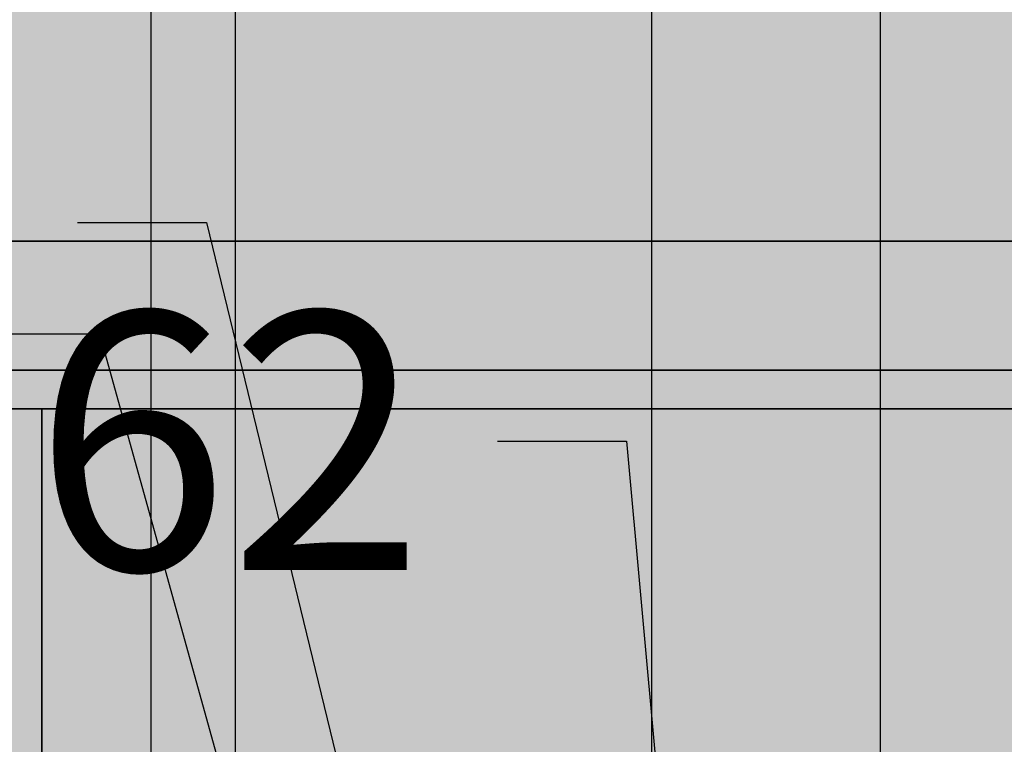
# Model space of a CAD drawing. Units: millimetres. Extents: x 130 to 1021, y 147 to 699.
# Tile 29 of 40: x 366 to 442, y 548 to 604. Entities that reach past the tile are written whole.
import ezdxf

# ---------------------------------------------------------------- set-up
doc = ezdxf.new("R2010")
doc.units = ezdxf.units.MM
doc.header["$MEASUREMENT"] = 0
for name, color, linetype, lineweight in [('A-ANNO-DIMS', 2, 'Continuous', 18), ('A-ELEV', 7, 'Continuous', 35), ('A-ELEV-PATT', 9, 'Continuous', 13)]:
    doc.layers.add(name, color=color, linetype=linetype, lineweight=lineweight)
doc.styles.get("Standard").update_dxf_attribs({"font": 'arial.ttf'})
doc.dimstyles.get("Standard").update_dxf_attribs({"dimtxt": 20, "dimasz": 10, "dimexe": 10, "dimexo": 10, "dimgap": 5, "dimtad": 0, "dimtih": 1, "dimtoh": 1, "dimdec": 0, "dimzin": 0, "dimdsep": 46, "dimtxsty": 'Standard', "dimcen": 5, "dimadec": 0, "dimazin": 0, "dimtfac": 1, "dimtdec": 0, "dimtofl": 0, "dimtmove": 0, "dimatfit": 3, "dimfxl": 1, "dimtolj": 1, "dimtzin": 0, "dimarcsym": 0})

# ---------------------------------------------------------------- blocks, each defined once
blk = doc.blocks.new('*D11')
at = {"layer": 'A-ANNO-DIMS', "color": 0, "lineweight": -2, "transparency": 16777216}
for p, q in [((737.374, 648.699), (737.374, 149.739)), ((299.374, 566.947), (299.374, 149.739)), ((309.374, 159.739), (490.857, 159.739)), ((727.374, 159.739), (545.891, 159.739))]:
    blk.add_line(p, q, dxfattribs=at)
at = {"layer": 'A-ANNO-DIMS', "color": 0, "transparency": 16777216}
for points in [[(309.374, 161.406), (309.374, 158.073), (299.374, 159.739)], [(727.374, 161.406), (727.374, 158.073), (737.374, 159.739)]]:
    blk.add_solid(points, dxfattribs=at)
at = {"layer": 'Defpoints', "color": 0, "transparency": 16777216}
for p in [(737.374, 658.699), (299.374, 576.947), (737.374, 159.739)]:
    blk.add_point(p, dxfattribs=at)
at = {"layer": 'A-ANNO-DIMS', "color": 0, "transparency": 16777216, "insert": (518.374, 159.739), "char_height": 20, "attachment_point": 5}
blk.add_mtext('\\A1;438', dxfattribs=at)
blk = doc.blocks.new('*D12')
at = {"layer": 'A-ANNO-DIMS', "color": 0, "lineweight": -2, "transparency": 16777216}
for p, q in [((477.374, 661.947), (265.074, 661.947)), ((275.074, 651.947), (275.074, 438.205)), ((275.074, 194.039), (275.074, 407.782)), ((357.163, 184.039), (265.074, 184.039))]:
    blk.add_line(p, q, dxfattribs=at)
at = {"layer": 'A-ANNO-DIMS', "color": 0, "transparency": 16777216}
for points in [[(273.407, 651.947), (276.74, 651.947), (275.074, 661.947)], [(273.407, 194.039), (276.74, 194.039), (275.074, 184.039)]]:
    blk.add_solid(points, dxfattribs=at)
at = {"layer": 'Defpoints', "color": 0, "transparency": 16777216}
for p in [(275.074, 661.947), (487.374, 661.947), (367.163, 184.039)]:
    blk.add_point(p, dxfattribs=at)
at = {"layer": 'A-ANNO-DIMS', "color": 0, "transparency": 16777216, "insert": (275.074, 422.993), "char_height": 20, "attachment_point": 5}
blk.add_mtext('\\A1;477.9', dxfattribs=at)
blk = doc.blocks.new('*D14')
at = {"layer": 'A-ANNO-DIMS', "color": 0, "lineweight": -2, "transparency": 16777216}
for p, q in [((307.374, 641.947), (307.374, 696.247)), ((327.374, 579.884), (327.374, 696.247)), ((297.374, 686.247), (287.374, 686.247)), ((337.374, 686.247), (347.374, 686.247))]:
    blk.add_line(p, q, dxfattribs=at)
at = {"layer": 'A-ANNO-DIMS', "color": 0, "transparency": 16777216}
for points in [[(297.374, 687.914), (297.374, 684.581), (307.374, 686.247)], [(337.374, 687.914), (337.374, 684.581), (327.374, 686.247)]]:
    blk.add_solid(points, dxfattribs=at)
at = {"layer": 'Defpoints', "color": 0, "transparency": 16777216}
for p in [(327.374, 686.247), (307.374, 631.947), (327.374, 569.884)]:
    blk.add_point(p, dxfattribs=at)
at = {"layer": 'A-ANNO-DIMS', "color": 0, "transparency": 16777216, "insert": (366.835, 686.247), "char_height": 20, "attachment_point": 5}
blk.add_mtext('\\A1;20', dxfattribs=at)
blk = doc.blocks.new('*D15')
at = {"layer": 'A-ANNO-DIMS', "color": 0, "lineweight": -2, "transparency": 16777216}
for p, q in [((327.374, 579.884), (327.374, 696.247)), ((357.941, 411.947), (357.941, 696.247)), ((337.374, 686.247), (347.941, 686.247)), ((357.941, 686.247), (367.941, 686.247))]:
    blk.add_line(p, q, dxfattribs=at)
at = {"layer": 'A-ANNO-DIMS', "color": 0, "transparency": 16777216}
for points in [[(337.374, 687.914), (337.374, 684.581), (327.374, 686.247)], [(347.941, 687.914), (347.941, 684.581), (357.941, 686.247)]]:
    blk.add_solid(points, dxfattribs=at)
at = {"layer": 'Defpoints', "color": 0, "transparency": 16777216}
for p in [(357.941, 686.247), (327.374, 569.884), (357.941, 401.947)]:
    blk.add_point(p, dxfattribs=at)
at = {"layer": 'A-ANNO-DIMS', "color": 0, "transparency": 16777216, "insert": (406.679, 686.247), "char_height": 20, "attachment_point": 5}
blk.add_mtext('\\A1;30.57', dxfattribs=at)
blk = doc.blocks.new('*D16')
at = {"layer": 'A-ANNO-DIMS', "color": 0, "lineweight": -2, "transparency": 16777216}
for p, q in [((357.941, 411.947), (357.941, 696.247)), ((363.922, 579.884), (363.922, 696.247)), ((347.941, 686.247), (337.941, 686.247)), ((373.922, 686.247), (383.922, 686.247))]:
    blk.add_line(p, q, dxfattribs=at)
at = {"layer": 'A-ANNO-DIMS', "color": 0, "transparency": 16777216}
for points in [[(347.941, 687.914), (347.941, 684.581), (357.941, 686.247)], [(373.922, 687.914), (373.922, 684.581), (363.922, 686.247)]]:
    blk.add_solid(points, dxfattribs=at)
at = {"layer": 'Defpoints', "color": 0, "transparency": 16777216}
for p in [(363.922, 686.247), (363.922, 569.884), (357.941, 401.947)]:
    blk.add_point(p, dxfattribs=at)
at = {"layer": 'A-ANNO-DIMS', "color": 0, "transparency": 16777216, "insert": (420.737, 686.247), "char_height": 20, "attachment_point": 5}
blk.add_mtext('\\A1;5.981', dxfattribs=at)
blk = doc.blocks.new('*D17')
at = {"layer": 'A-ANNO-DIMS', "color": 0, "lineweight": -2, "transparency": 16777216}
for p, q in [((363.922, 579.884), (363.922, 696.247)), ((375.85, 490.216), (375.85, 696.247)), ((353.922, 686.247), (343.922, 686.247)), ((385.85, 686.247), (395.85, 686.247))]:
    blk.add_line(p, q, dxfattribs=at)
at = {"layer": 'A-ANNO-DIMS', "color": 0, "transparency": 16777216}
for points in [[(353.922, 687.914), (353.922, 684.581), (363.922, 686.247)], [(385.85, 687.914), (385.85, 684.581), (375.85, 686.247)]]:
    blk.add_solid(points, dxfattribs=at)
at = {"layer": 'Defpoints', "color": 0, "transparency": 16777216}
for p in [(375.85, 686.247), (363.922, 569.884), (375.85, 480.216)]:
    blk.add_point(p, dxfattribs=at)
at = {"layer": 'A-ANNO-DIMS', "color": 0, "transparency": 16777216, "insert": (441.444, 686.247), "char_height": 20, "attachment_point": 5}
blk.add_mtext('\\A1;11.928', dxfattribs=at)
blk = doc.blocks.new('*D18')
at = {"layer": 'A-ANNO-DIMS', "color": 0, "lineweight": -2, "transparency": 16777216}
for p, q in [((375.85, 490.216), (375.85, 696.247)), ((382.374, 388.947), (382.374, 696.247)), ((365.85, 686.247), (355.85, 686.247)), ((392.374, 686.247), (402.374, 686.247))]:
    blk.add_line(p, q, dxfattribs=at)
at = {"layer": 'A-ANNO-DIMS', "color": 0, "transparency": 16777216}
for points in [[(365.85, 687.914), (365.85, 684.581), (375.85, 686.247)], [(392.374, 687.914), (392.374, 684.581), (382.374, 686.247)]]:
    blk.add_solid(points, dxfattribs=at)
at = {"layer": 'Defpoints', "color": 0, "transparency": 16777216}
for p in [(382.374, 686.247), (375.85, 480.216), (382.374, 378.947)]:
    blk.add_point(p, dxfattribs=at)
at = {"layer": 'A-ANNO-DIMS', "color": 0, "transparency": 16777216, "insert": (441.132, 686.247), "char_height": 20, "attachment_point": 5}
blk.add_mtext('\\A1;6.524', dxfattribs=at)
blk = doc.blocks.new('*D19')
at = {"layer": 'A-ANNO-DIMS', "color": 0, "lineweight": -2, "transparency": 16777216}
for p, q in [((382.374, 388.947), (382.374, 696.247)), ((414.652, 510.881), (414.652, 696.247)), ((392.374, 686.247), (404.652, 686.247)), ((414.652, 686.247), (424.652, 686.247))]:
    blk.add_line(p, q, dxfattribs=at)
at = {"layer": 'A-ANNO-DIMS', "color": 0, "transparency": 16777216}
for points in [[(392.374, 687.914), (392.374, 684.581), (382.374, 686.247)], [(404.652, 687.914), (404.652, 684.581), (414.652, 686.247)]]:
    blk.add_solid(points, dxfattribs=at)
at = {"layer": 'Defpoints', "color": 0, "transparency": 16777216}
for p in [(414.652, 686.247), (414.652, 500.881), (382.374, 378.947)]:
    blk.add_point(p, dxfattribs=at)
at = {"layer": 'A-ANNO-DIMS', "color": 0, "transparency": 16777216, "insert": (463.411, 686.247), "char_height": 20, "attachment_point": 5}
blk.add_mtext('\\A1;32.28', dxfattribs=at)
blk = doc.blocks.new('*D20')
at = {"layer": 'A-ANNO-DIMS', "color": 0, "lineweight": -2, "transparency": 16777216}
for p, q in [((414.652, 510.881), (414.652, 696.247)), ((432.374, 388.947), (432.374, 696.247)), ((404.652, 686.247), (394.652, 686.247)), ((442.374, 686.247), (452.374, 686.247))]:
    blk.add_line(p, q, dxfattribs=at)
at = {"layer": 'A-ANNO-DIMS', "color": 0, "transparency": 16777216}
for points in [[(404.652, 687.914), (404.652, 684.581), (414.652, 686.247)], [(442.374, 687.914), (442.374, 684.581), (432.374, 686.247)]]:
    blk.add_solid(points, dxfattribs=at)
at = {"layer": 'Defpoints', "color": 0, "transparency": 16777216}
for p in [(432.374, 686.247), (414.652, 500.881), (432.374, 378.947)]:
    blk.add_point(p, dxfattribs=at)
at = {"layer": 'A-ANNO-DIMS', "color": 0, "transparency": 16777216, "insert": (490.075, 686.247), "char_height": 20, "attachment_point": 5}
blk.add_mtext('\\A1;17.72', dxfattribs=at)
blk = doc.blocks.new('*D21')
at = {"layer": 'A-ANNO-DIMS', "color": 0, "lineweight": -2, "transparency": 16777216}
for p, q in [((432.374, 388.947), (432.374, 696.247)), ((447.374, 656.947), (447.374, 696.247)), ((422.374, 686.247), (412.374, 686.247)), ((457.374, 686.247), (467.374, 686.247))]:
    blk.add_line(p, q, dxfattribs=at)
at = {"layer": 'A-ANNO-DIMS', "color": 0, "transparency": 16777216}
for points in [[(422.374, 687.914), (422.374, 684.581), (432.374, 686.247)], [(457.374, 687.914), (457.374, 684.581), (447.374, 686.247)]]:
    blk.add_solid(points, dxfattribs=at)
at = {"layer": 'Defpoints', "color": 0, "transparency": 16777216}
for p in [(447.374, 686.247), (447.374, 646.947), (432.374, 378.947)]:
    blk.add_point(p, dxfattribs=at)
at = {"layer": 'A-ANNO-DIMS', "color": 0, "transparency": 16777216, "insert": (485.832, 686.247), "char_height": 20, "attachment_point": 5}
blk.add_mtext('\\A1;15', dxfattribs=at)
blk = doc.blocks.new('*D22')
at = {"layer": 'A-ANNO-DIMS', "color": 0, "lineweight": -2, "transparency": 16777216}
for p, q in [((447.374, 656.947), (447.374, 696.247)), ((466.767, 403.947), (466.767, 696.247)), ((437.374, 686.247), (427.374, 686.247)), ((476.767, 686.247), (486.767, 686.247))]:
    blk.add_line(p, q, dxfattribs=at)
at = {"layer": 'A-ANNO-DIMS', "color": 0, "transparency": 16777216}
for points in [[(437.374, 687.914), (437.374, 684.581), (447.374, 686.247)], [(476.767, 687.914), (476.767, 684.581), (466.767, 686.247)]]:
    blk.add_solid(points, dxfattribs=at)
at = {"layer": 'Defpoints', "color": 0, "transparency": 16777216}
for p in [(466.767, 686.247), (447.374, 646.947), (466.767, 393.947)]:
    blk.add_point(p, dxfattribs=at)
at = {"layer": 'A-ANNO-DIMS', "color": 0, "transparency": 16777216, "insert": (532.34, 686.247), "char_height": 20, "attachment_point": 5}
blk.add_mtext('\\A1;19.393', dxfattribs=at)
blk = doc.blocks.new('*D44')
at = {"layer": 'A-ANNO-DIMS', "color": 0, "lineweight": -2, "transparency": 16777216}
for p, q in [((317.374, 569.884), (265.074, 569.884)), ((275.074, 559.884), (275.074, 550.594)), ((275.074, 510.881), (275.074, 520.171)), ((404.652, 500.881), (265.074, 500.881))]:
    blk.add_line(p, q, dxfattribs=at)
at = {"layer": 'A-ANNO-DIMS', "color": 0, "transparency": 16777216}
for points in [[(273.407, 559.884), (276.74, 559.884), (275.074, 569.884)], [(273.407, 510.881), (276.74, 510.881), (275.074, 500.881)]]:
    blk.add_solid(points, dxfattribs=at)
at = {"layer": 'Defpoints', "color": 0, "transparency": 16777216}
for p in [(275.074, 569.884), (327.374, 569.884), (414.652, 500.881)]:
    blk.add_point(p, dxfattribs=at)
at = {"layer": 'A-ANNO-DIMS', "color": 0, "transparency": 16777216, "insert": (275.074, 535.383), "char_height": 20, "attachment_point": 5}
blk.add_mtext('\\A1;69', dxfattribs=at)
blk = doc.blocks.new('*D66')
at = {"layer": 'A-ANNO-DIMS', "color": 0, "lineweight": -2, "transparency": 16777216}
for p, q in [((341.579, 557.194), (351.579, 557.194)), ((351.579, 557.194), (376.947, 478.135)), ((427.374, 315.978), (427.374, 325.978)), ((422.374, 320.978), (432.374, 320.978))]:
    blk.add_line(p, q, dxfattribs=at)
at = {"layer": 'A-ANNO-DIMS', "color": 0, "transparency": 16777216}
blk.add_solid([(378.534, 478.644), (375.36, 477.626), (380.002, 468.613)], dxfattribs=at)
at = {"layer": 'Defpoints', "color": 0, "transparency": 16777216}
for p in [(380.002, 468.613), (427.374, 320.978)]:
    blk.add_point(p, dxfattribs=at)
at = {"layer": 'A-ANNO-DIMS', "color": 0, "transparency": 16777216, "insert": (263.53, 557.194), "char_height": 20, "attachment_point": 5}
blk.add_mtext('\\A1;4X R155.05', dxfattribs=at)
blk = doc.blocks.new('*D68')
at = {"layer": 'A-ANNO-DIMS', "color": 0, "lineweight": -2, "transparency": 16777216}
for p, q in [((361.841, 579.756), (371.841, 579.756)), ((371.841, 579.756), (392.167, 506.693)), ((433.191, 354.23), (433.191, 364.23)), ((428.191, 359.23), (438.191, 359.23))]:
    blk.add_line(p, q, dxfattribs=at)
at = {"layer": 'A-ANNO-DIMS', "color": 0, "transparency": 16777216}
blk.add_solid([(393.773, 507.14), (390.561, 506.246), (394.847, 497.059)], dxfattribs=at)
at = {"layer": 'Defpoints', "color": 0, "transparency": 16777216}
for p in [(394.847, 497.059), (433.191, 359.23)]:
    blk.add_point(p, dxfattribs=at)
at = {"layer": 'A-ANNO-DIMS', "color": 0, "transparency": 16777216, "insert": (305.764, 579.756), "char_height": 20, "attachment_point": 5}
blk.add_mtext('\\A1;R143.06', dxfattribs=at)
blk = doc.blocks.new('*D69')
at = {"layer": 'A-ANNO-DIMS', "color": 0, "lineweight": -2, "transparency": 16777216}
for p, q in [((507.746, 572.261), (483.091, 501.813)), ((517.746, 572.261), (507.746, 572.261)), ((433.191, 354.23), (433.191, 364.23)), ((428.191, 359.23), (438.191, 359.23))]:
    blk.add_line(p, q, dxfattribs=at)
at = {"layer": 'A-ANNO-DIMS', "color": 0, "transparency": 16777216}
blk.add_solid([(481.518, 502.363), (484.664, 501.262), (479.788, 492.374)], dxfattribs=at)
at = {"layer": 'Defpoints', "color": 0, "transparency": 16777216}
for p in [(479.788, 492.374), (433.191, 359.23)]:
    blk.add_point(p, dxfattribs=at)
at = {"layer": 'A-ANNO-DIMS', "color": 0, "transparency": 16777216, "insert": (573.824, 572.261), "char_height": 20, "attachment_point": 5}
blk.add_mtext('\\A1;R141.06', dxfattribs=at)
blk = doc.blocks.new('*D70')
at = {"layer": 'A-ANNO-DIMS', "color": 0, "lineweight": -2, "transparency": 16777216}
for p, q in [((370.141, 588.4), (380.141, 588.4)), ((380.141, 588.4), (397.473, 517.008)), ((432.65, 367.109), (432.65, 377.109)), ((427.65, 372.109), (437.65, 372.109))]:
    blk.add_line(p, q, dxfattribs=at)
at = {"layer": 'A-ANNO-DIMS', "color": 0, "transparency": 16777216}
blk.add_solid([(399.093, 517.402), (395.854, 516.615), (399.832, 507.291)], dxfattribs=at)
at = {"layer": 'Defpoints', "color": 0, "transparency": 16777216}
for p in [(399.832, 507.291), (432.65, 372.109)]:
    blk.add_point(p, dxfattribs=at)
at = {"layer": 'A-ANNO-DIMS', "color": 0, "transparency": 16777216, "insert": (323.757, 588.4), "char_height": 20, "attachment_point": 5}
blk.add_mtext('\\A1;R139.1', dxfattribs=at)
blk = doc.blocks.new('*D71')
at = {"layer": 'A-ANNO-DIMS', "color": 0, "lineweight": -2, "transparency": 16777216}
for p, q in [((492.108, 581.609), (472.542, 512.666)), ((502.108, 581.609), (492.108, 581.609)), ((432.65, 367.109), (432.65, 377.109)), ((427.65, 372.109), (437.65, 372.109))]:
    blk.add_line(p, q, dxfattribs=at)
at = {"layer": 'A-ANNO-DIMS', "color": 0, "transparency": 16777216}
blk.add_solid([(470.938, 513.121), (474.145, 512.211), (469.812, 503.046)], dxfattribs=at)
at = {"layer": 'Defpoints', "color": 0, "transparency": 16777216}
for p in [(469.812, 503.046), (432.65, 372.109)]:
    blk.add_point(p, dxfattribs=at)
at = {"layer": 'A-ANNO-DIMS', "color": 0, "transparency": 16777216, "insert": (548.493, 581.609), "char_height": 20, "attachment_point": 5}
blk.add_mtext('\\A1;R136.1', dxfattribs=at)
blk = doc.blocks.new('*D72')
at = {"layer": 'A-ANNO-DIMS', "color": 0, "lineweight": -2, "transparency": 16777216}
for p, q in [((460.658, 573.64), (451.279, 503.49)), ((470.658, 573.64), (460.658, 573.64)), ((432.115, 355.142), (432.115, 365.142)), ((427.115, 360.142), (437.115, 360.142))]:
    blk.add_line(p, q, dxfattribs=at)
at = {"layer": 'A-ANNO-DIMS', "color": 0, "transparency": 16777216}
blk.add_solid([(449.628, 503.711), (452.931, 503.27), (449.954, 493.579)], dxfattribs=at)
at = {"layer": 'Defpoints', "color": 0, "transparency": 16777216}
for p in [(449.954, 493.579), (432.115, 360.142)]:
    blk.add_point(p, dxfattribs=at)
at = {"layer": 'A-ANNO-DIMS', "color": 0, "transparency": 16777216, "insert": (526.64, 573.64), "char_height": 20, "attachment_point": 5}
blk.add_mtext('\\A1;R134.62', dxfattribs=at)
blk = doc.blocks.new('*D73')
at = {"layer": 'A-ANNO-DIMS', "color": 0, "lineweight": -2, "transparency": 16777216}
for p, q in [((402.678, 571.448), (412.678, 571.448)), ((412.678, 571.448), (419.051, 502.166)), ((432.115, 355.142), (432.115, 365.142)), ((427.115, 360.142), (437.115, 360.142))]:
    blk.add_line(p, q, dxfattribs=at)
at = {"layer": 'A-ANNO-DIMS', "color": 0, "transparency": 16777216}
blk.add_solid([(420.711, 502.319), (417.391, 502.014), (419.967, 492.208)], dxfattribs=at)
at = {"layer": 'Defpoints', "color": 0, "transparency": 16777216}
for p in [(419.967, 492.208), (432.115, 360.142)]:
    blk.add_point(p, dxfattribs=at)
at = {"layer": 'A-ANNO-DIMS', "color": 0, "transparency": 16777216, "insert": (346.696, 571.448), "char_height": 20, "attachment_point": 5}
blk.add_mtext('\\A1;R132.62', dxfattribs=at)

msp = doc.modelspace()

# ---------------------------------------------------------------- hatches: boundary and pattern name
at = {"layer": 'A-ELEV-PATT'}
h = msp.add_hatch(color=256, dxfattribs=at)
h.dxf.hatch_style = 1
h.paths.add_polyline_path([(737.3738, 658.6988, 0.0135961), (632.4019, 661.9473), (607.3738, 661.9473), (487.3738, 661.9473), (487.3738, 649.9473), (607.3738, 649.9473), (632.3794, 649.9473, -0.0136841), (737.3738, 646.6784)])
h.paths.add_polyline_path([(732.3738, 643.9599, 0.0130529), (632.3738, 646.9473), (607.3738, 646.9473), (487.3738, 646.9473), (487.3738, 596.9473), (632.3738, 596.9473, -0.0130529), (732.3738, 593.9599)])
h.paths.add_polyline_path([(737.3738, 593.6732, 0.0137063), (632.3738, 596.9473), (487.3738, 596.9473), (487.3738, 586.9473), (632.355, 586.9473, -0.0137808), (737.3738, 583.6559)])
h.paths.add_polyline_path([(447.3738, 646.9473), (307.3738, 646.9473), (302.3738, 646.9473), (302.3738, 634.9473), (447.3738, 634.9473)])
h.paths.add_polyline_path([(447.3738, 631.9473), (307.3738, 631.9473), (307.3738, 586.9473), (447.3738, 586.9473)])
h.paths.add_polyline_path([(447.3738, 586.9473), (307.3738, 586.9473), (302.3738, 586.9473), (302.3738, 576.9473), (447.3738, 576.9473)])
h.paths.add_polyline_path([(447.3738, 573.9473), (367.3738, 573.9473), (367.3738, 539.9473), (447.3738, 539.9473)])
h.paths.add_polyline_path([(447.3738, 537.9473), (367.3738, 537.9473), (367.3738, 507.9473), (400.392, 507.4253, -0.001728), (401.3281, 507.6451, -0.5220025), (425.6117, 511.0391, -0.0391849), (447.3738, 510.4359), (447.3738, 510.7883)])
h.paths.add_polyline_path([(394.7238, 505.9473), (367.3738, 505.9473), (367.3738, 476.9473, -0.0146512), (375.8501, 480.2159), (376.1506, 499.2266, -0.0355419)])
h.paths.add_polyline_path([(632.3738, 583.9473), (552.3738, 583.9473), (552.3738, 550.9473), (632.3738, 550.9473)])
h.paths.add_polyline_path([(632.3738, 548.9473), (552.3738, 548.9473), (552.3738, 515.9473), (632.3738, 515.9473)])
h.paths.add_polyline_path([(632.3738, 513.9473), (552.3738, 513.9473), (552.3738, 476.9473), (632.3738, 476.9473)])
h.paths.add_polyline_path([(737.3738, 473.6903, 0.0136326), (632.3926, 476.9473), (552.3738, 476.9473), (487.3738, 476.9473), (487.3738, 466.9473), (632.3738, 466.9473, -0.0137063), (737.3738, 463.6732)])
h.paths.add_polyline_path([(732.3738, 460.9552, 0.0130741), (632.3681, 463.9473), (487.3738, 463.9473), (487.3738, 407.735, -0.0032286), (489.3544, 406.9473), (632.3926, 406.9473, -0.0129826), (732.3738, 403.9755)])
h.paths.add_polyline_path([(487.3738, 463.9473, 0.20133), (367.3738, 463.9473), (367.3738, 407.735, -0.1882031), (487.3738, 407.735)])
h.paths.add_polyline_path([(367.3738, 476.9473), (367.3738, 466.9473, -0.2013309), (487.3738, 466.9473), (487.3738, 476.9473, 0.20133)])
h.paths.add_polyline_path([(367.3738, 463.9473), (307.3738, 463.9473), (307.3738, 401.9473), (357.9413, 401.9473), (367.3738, 407.735)])
h.paths.add_polyline_path([(367.3738, 476.9473), (302.3738, 476.9473), (302.3738, 466.9473), (367.3738, 466.9473)])
h.paths.add_polyline_path([(632.8184, 366.9453), (552.3738, 366.9453), (552.3738, 393.9473), (632.8184, 393.9473)])
h.paths.add_polyline_path([(632.8184, 357.2114), (632.8184, 363.9453), (552.3738, 363.9453), (552.3738, 357.2114), (552.3738, 336.9453), (632.8184, 336.9453)])
h.paths.add_polyline_path([(632.8184, 333.9453), (552.3738, 333.9453), (552.3738, 306.9453), (632.8184, 306.9453)])
h.paths.add_polyline_path([(632.8184, 303.9453), (552.3738, 303.9453), (552.3738, 273.9473), (632.355, 273.9473, 0.0000608), (632.8184, 273.9491)])
h.paths.add_polyline_path([(737.3738, 403.6903, 0.0136326), (632.3926, 406.9473), (489.3544, 406.9473, 0.1915481), (367.3738, 407.735), (367.3738, 396.9473, -0.2013309), (487.3738, 396.9473), (632.3738, 396.9473, -0.0137063), (737.3738, 393.6732)])
h.paths.add_polyline_path([(357.9413, 401.9473), (307.3738, 401.9473), (307.3738, 391.9473), (357.9413, 391.9473)])
h.paths.add_polyline_path([(357.9413, 357.2114), (357.9413, 388.9473), (307.3738, 388.9473), (307.3738, 357.2114), (307.3738, 273.9473), (357.9413, 273.9473)])
h.paths.add_polyline_path([(732.3738, 263.93, -0.0130317), (632.3794, 260.9473), (466.7667, 260.9473), (466.7667, 240.9473), (469.8406, 236.978), (469.8406, 221.978), (472.9145, 218.0087), (472.9145, 213.9473), (607.3738, 213.9473), (732.3738, 213.9473)])
h.paths.add_polyline_path([(732.3738, 290.889), (722.479, 290.889), (722.479, 301.889), (732.3738, 301.889), (732.3738, 305.889), (722.479, 305.889), (722.479, 316.889), (732.3738, 316.889), (732.3738, 320.889), (722.479, 320.889), (722.479, 331.889), (732.3738, 331.889), (732.3738, 335.889), (722.479, 335.889), (722.479, 346.889), (732.3738, 346.889), (732.3738, 350.889), (722.479, 350.889), (722.479, 361.889), (732.3738, 361.889), (732.3738, 365.889), (722.479, 365.889), (722.479, 376.889), (732.3738, 376.889), (732.3738, 380.889), (722.479, 380.889), (722.479, 391.4848, 0.0005233), (718.479, 391.6843), (718.479, 380.889), (707.479, 380.889), (707.479, 392.1896, 0.0005231), (703.479, 392.3576), (703.479, 380.889), (692.479, 380.889), (692.479, 392.7765, 0.0005229), (688.479, 392.9131), (688.479, 380.889), (677.479, 380.889), (677.479, 393.2456, 0.0005228), (673.479, 393.3508), (673.479, 380.889), (662.479, 380.889), (662.479, 393.597, 0.0005227), (658.479, 393.6709), (658.479, 380.889), (647.479, 380.889), (647.479, 393.8308, 0.0005226), (643.479, 393.8732), (643.479, 380.889), (632.8184, 380.889), (632.8184, 376.889), (643.479, 376.889), (643.479, 365.889), (632.8184, 365.889), (632.8184, 361.889), (643.479, 361.889), (643.479, 350.889), (632.8184, 350.889), (632.8184, 346.889), (643.479, 346.889), (643.479, 335.889), (632.8184, 335.889), (632.8184, 331.889), (643.479, 331.889), (643.479, 320.889), (632.8184, 320.889), (632.8184, 316.889), (643.479, 316.889), (643.479, 305.889), (632.8184, 305.889), (632.8184, 301.889), (643.479, 301.889), (643.479, 290.889), (632.8184, 290.889), (632.8184, 286.889), (643.479, 286.889), (643.479, 274.0217, 0.0005246), (647.479, 274.0643), (647.479, 286.889), (658.479, 286.889), (658.479, 274.2248, 0.0005246), (662.479, 274.2989), (662.479, 286.889), (673.479, 286.889), (673.479, 274.546, 0.0005247), (677.479, 274.6516), (677.479, 286.889), (688.479, 286.889), (688.479, 274.9853, 0.0005248), (692.479, 275.1224), (692.479, 286.889), (703.479, 286.889), (703.479, 275.5429, 0.000525), (707.479, 275.7115), (707.479, 286.889), (718.479, 286.889), (718.479, 276.2187, 0.0005252), (722.479, 276.4189), (722.479, 286.889), (732.3738, 286.889)])
h.paths.add_polyline_path([(718.479, 290.889), (707.479, 290.889), (707.479, 301.889), (718.479, 301.889)], flags=16)
h.paths.add_polyline_path([(703.479, 290.889), (692.479, 290.889), (692.479, 301.889), (703.479, 301.889)], flags=16)
h.paths.add_polyline_path([(718.479, 305.889), (707.479, 305.889), (707.479, 316.889), (718.479, 316.889)], flags=16)
h.paths.add_polyline_path([(703.479, 305.889), (692.479, 305.889), (692.479, 316.889), (703.479, 316.889)], flags=16)
h.paths.add_polyline_path([(688.479, 290.889), (677.479, 290.889), (677.479, 301.889), (688.479, 301.889)], flags=16)
h.paths.add_polyline_path([(718.479, 320.889), (707.479, 320.889), (707.479, 331.889), (718.479, 331.889)], flags=16)
h.paths.add_polyline_path([(688.479, 305.889), (677.479, 305.889), (677.479, 316.889), (688.479, 316.889)], flags=16)
h.paths.add_polyline_path([(703.479, 320.889), (692.479, 320.889), (692.479, 331.889), (703.479, 331.889)], flags=16)
h.paths.add_polyline_path([(688.479, 320.889), (677.479, 320.889), (677.479, 331.889), (688.479, 331.889)], flags=16)
h.paths.add_polyline_path([(673.479, 290.889), (662.479, 290.889), (662.479, 301.889), (673.479, 301.889)], flags=16)
h.paths.add_polyline_path([(718.479, 335.889), (707.479, 335.889), (707.479, 346.889), (718.479, 346.889)], flags=16)
h.paths.add_polyline_path([(673.479, 305.889), (662.479, 305.889), (662.479, 316.889), (673.479, 316.889)], flags=16)
h.paths.add_polyline_path([(703.479, 335.889), (692.479, 335.889), (692.479, 346.889), (703.479, 346.889)], flags=16)
h.paths.add_polyline_path([(673.479, 320.889), (662.479, 320.889), (662.479, 331.889), (673.479, 331.889)], flags=16)
h.paths.add_polyline_path([(688.479, 335.889), (677.479, 335.889), (677.479, 346.889), (688.479, 346.889)], flags=16)
h.paths.add_polyline_path([(658.479, 290.889), (647.479, 290.889), (647.479, 301.889), (658.479, 301.889)], flags=16)
h.paths.add_polyline_path([(718.479, 350.889), (707.479, 350.889), (707.479, 361.889), (718.479, 361.889)], flags=16)
h.paths.add_polyline_path([(658.479, 305.889), (647.479, 305.889), (647.479, 316.889), (658.479, 316.889)], flags=16)
h.paths.add_polyline_path([(703.479, 350.889), (692.479, 350.889), (692.479, 361.889), (703.479, 361.889)], flags=16)
h.paths.add_polyline_path([(673.479, 335.889), (662.479, 335.889), (662.479, 346.889), (673.479, 346.889)], flags=16)
h.paths.add_polyline_path([(658.479, 320.889), (647.479, 320.889), (647.479, 331.889), (658.479, 331.889)], flags=16)
h.paths.add_polyline_path([(688.479, 350.889), (677.479, 350.889), (677.479, 361.889), (688.479, 361.889)], flags=16)
h.paths.add_polyline_path([(718.479, 365.889), (707.479, 365.889), (707.479, 376.889), (718.479, 376.889)], flags=16)
h.paths.add_polyline_path([(658.479, 335.889), (647.479, 335.889), (647.479, 346.889), (658.479, 346.889)], flags=16)
h.paths.add_polyline_path([(673.479, 350.889), (662.479, 350.889), (662.479, 361.889), (673.479, 361.889)], flags=16)
h.paths.add_polyline_path([(703.479, 365.889), (692.479, 365.889), (692.479, 376.889), (703.479, 376.889)], flags=16)
h.paths.add_polyline_path([(688.479, 365.889), (677.479, 365.889), (677.479, 376.889), (688.479, 376.889)], flags=16)
h.paths.add_polyline_path([(658.479, 350.889), (647.479, 350.889), (647.479, 361.889), (658.479, 361.889)], flags=16)
h.paths.add_polyline_path([(673.479, 365.889), (662.479, 365.889), (662.479, 376.889), (673.479, 376.889)], flags=16)
h.paths.add_polyline_path([(658.479, 365.889), (647.479, 365.889), (647.479, 376.889), (658.479, 376.889)], flags=16)
h.paths.add_polyline_path([(732.3738, 503.9786), (722.3392, 503.9786), (722.3392, 514.9786), (732.3738, 514.9786), (732.3738, 518.9786), (722.3392, 518.9786), (722.3392, 529.9786), (732.3738, 529.9786), (732.3738, 533.9786), (722.3392, 533.9786), (722.3392, 544.9786), (732.3738, 544.9786), (732.3738, 546.9473), (732.3738, 548.9786), (722.3392, 548.9786), (722.3392, 559.9786), (732.3738, 559.9786), (732.3738, 563.9786), (722.3392, 563.9786), (722.3392, 574.9786), (732.3738, 574.9786), (732.3738, 578.9786), (722.3392, 578.9786), (722.3392, 581.4789, 0.000526), (718.3392, 581.6791), (718.3392, 578.9786), (707.3392, 578.9786), (707.3392, 582.1863, 0.0005258), (703.3392, 582.355), (703.3392, 578.9786), (692.3392, 578.9786), (692.3392, 582.7752, 0.0005257), (688.3392, 582.9123), (688.3392, 578.9786), (677.3392, 578.9786), (677.3392, 583.2457, 0.0005255), (673.3392, 583.3512), (673.3392, 578.9786), (662.3392, 578.9786), (662.3392, 583.5978, 0.0005254), (658.3392, 583.6718), (658.3392, 578.9786), (647.3392, 578.9786), (647.3392, 583.8317, 0.0005254), (643.3392, 583.8741), (643.3392, 578.9786), (632.3738, 578.9786), (632.3738, 574.9786), (643.3392, 574.9786), (643.3392, 563.9786), (632.3738, 563.9786), (632.3738, 559.9786), (643.3392, 559.9786), (643.3392, 548.9786), (632.3738, 548.9786), (632.3738, 544.9786), (643.3392, 544.9786), (643.3392, 533.9786), (632.3738, 533.9786), (632.3738, 529.9786), (643.3392, 529.9786), (643.3392, 518.9786), (632.3738, 518.9786), (632.3738, 515.9473), (632.3738, 514.9786), (643.3392, 514.9786), (643.3392, 503.9786), (632.3738, 503.9786), (632.3738, 499.9786), (643.3392, 499.9786), (643.3392, 488.9786), (632.3738, 488.9786), (632.3738, 484.9786), (643.3392, 484.9786), (643.3392, 476.8751, -0.0005191), (647.3392, 476.8332), (647.3392, 484.9786), (658.3392, 484.9786), (658.3392, 476.6752, -0.0005192), (662.3392, 476.6022), (662.3392, 484.9786), (673.3392, 484.9786), (673.3392, 476.3585, -0.0005193), (677.3392, 476.2543), (677.3392, 484.9786), (688.3392, 484.9786), (688.3392, 475.9248, -0.0005194), (692.3392, 475.7894), (692.3392, 484.9786), (703.3392, 484.9786), (703.3392, 475.3741, -0.0005195), (707.3392, 475.2075), (707.3392, 484.9786), (718.3392, 484.9786), (718.3392, 474.7064, -0.0005197), (722.3392, 474.5086), (722.3392, 484.9786), (732.3738, 484.9786), (732.3738, 488.9786), (722.3392, 488.9786), (722.3392, 499.9786), (732.3738, 499.9786)])
h.paths.add_polyline_path([(718.3392, 503.9786), (707.3392, 503.9786), (707.3392, 514.9786), (718.3392, 514.9786)], flags=16)
h.paths.add_polyline_path([(718.3392, 499.9786), (718.3392, 488.9786), (707.3392, 488.9786), (707.3392, 499.9786)], flags=16)
h.paths.add_polyline_path([(718.3392, 518.9786), (707.3392, 518.9786), (707.3392, 529.9786), (718.3392, 529.9786)], flags=16)
h.paths.add_polyline_path([(703.3392, 503.9786), (692.3392, 503.9786), (692.3392, 514.9786), (703.3392, 514.9786)], flags=16)
h.paths.add_polyline_path([(703.3392, 499.9786), (703.3392, 488.9786), (692.3392, 488.9786), (692.3392, 499.9786)], flags=16)
h.paths.add_polyline_path([(703.3392, 518.9786), (692.3392, 518.9786), (692.3392, 529.9786), (703.3392, 529.9786)], flags=16)
h.paths.add_polyline_path([(718.3392, 533.9786), (707.3392, 533.9786), (707.3392, 544.9786), (718.3392, 544.9786)], flags=16)
h.paths.add_polyline_path([(688.3392, 503.9786), (677.3392, 503.9786), (677.3392, 514.9786), (688.3392, 514.9786)], flags=16)
h.paths.add_polyline_path([(688.3392, 499.9786), (688.3392, 488.9786), (677.3392, 488.9786), (677.3392, 499.9786)], flags=16)
h.paths.add_polyline_path([(703.3392, 533.9786), (692.3392, 533.9786), (692.3392, 544.9786), (703.3392, 544.9786)], flags=16)
h.paths.add_polyline_path([(688.3392, 518.9786), (677.3392, 518.9786), (677.3392, 529.9786), (688.3392, 529.9786)], flags=16)
h.paths.add_polyline_path([(688.3392, 533.9786), (677.3392, 533.9786), (677.3392, 544.9786), (688.3392, 544.9786)], flags=16)
h.paths.add_polyline_path([(718.3392, 548.9786), (707.3392, 548.9786), (707.3392, 559.9786), (718.3392, 559.9786)], flags=16)
h.paths.add_polyline_path([(673.3392, 503.9786), (662.3392, 503.9786), (662.3392, 514.9786), (673.3392, 514.9786)], flags=16)
h.paths.add_polyline_path([(673.3392, 499.9786), (673.3392, 488.9786), (662.3392, 488.9786), (662.3392, 499.9786)], flags=16)
h.paths.add_polyline_path([(703.3392, 548.9786), (692.3392, 548.9786), (692.3392, 559.9786), (703.3392, 559.9786)], flags=16)
h.paths.add_polyline_path([(673.3392, 518.9786), (662.3392, 518.9786), (662.3392, 529.9786), (673.3392, 529.9786)], flags=16)
h.paths.add_polyline_path([(688.3392, 548.9786), (677.3392, 548.9786), (677.3392, 559.9786), (688.3392, 559.9786)], flags=16)
h.paths.add_polyline_path([(673.3392, 533.9786), (662.3392, 533.9786), (662.3392, 544.9786), (673.3392, 544.9786)], flags=16)
h.paths.add_polyline_path([(718.3392, 563.9786), (707.3392, 563.9786), (707.3392, 574.9786), (718.3392, 574.9786)], flags=16)
h.paths.add_polyline_path([(658.3392, 503.9786), (647.3392, 503.9786), (647.3392, 514.9786), (658.3392, 514.9786)], flags=16)
h.paths.add_polyline_path([(658.3392, 499.9786), (658.3392, 488.9786), (647.3392, 488.9786), (647.3392, 499.9786)], flags=16)
h.paths.add_polyline_path([(703.3392, 563.9786), (692.3392, 563.9786), (692.3392, 574.9786), (703.3392, 574.9786)], flags=16)
h.paths.add_polyline_path([(658.3392, 518.9786), (647.3392, 518.9786), (647.3392, 529.9786), (658.3392, 529.9786)], flags=16)
h.paths.add_polyline_path([(673.3392, 548.9786), (662.3392, 548.9786), (662.3392, 559.9786), (673.3392, 559.9786)], flags=16)
h.paths.add_polyline_path([(688.3392, 563.9786), (677.3392, 563.9786), (677.3392, 574.9786), (688.3392, 574.9786)], flags=16)
h.paths.add_polyline_path([(658.3392, 533.9786), (647.3392, 533.9786), (647.3392, 544.9786), (658.3392, 544.9786)], flags=16)
h.paths.add_polyline_path([(673.3392, 563.9786), (662.3392, 563.9786), (662.3392, 574.9786), (673.3392, 574.9786)], flags=16)
h.paths.add_polyline_path([(658.3392, 548.9786), (647.3392, 548.9786), (647.3392, 559.9786), (658.3392, 559.9786)], flags=16)
h.paths.add_polyline_path([(658.3392, 563.9786), (647.3392, 563.9786), (647.3392, 574.9786), (658.3392, 574.9786)], flags=16)
h = msp.add_hatch(color=256, dxfattribs=at)
h.dxf.hatch_style = 1
h.paths.add_polyline_path([(447.3738, 576.9473), (302.3738, 576.9473), (302.3738, 573.9473), (447.3738, 573.9473)])
h.paths.add_polyline_path([(487.3738, 583.9473), (487.3738, 586.9473), (447.3738, 576.9473), (447.3738, 573.9473)])
h.paths.add_polyline_path([(632.355, 586.9473), (487.3738, 586.9473), (487.3738, 583.9473), (632.3738, 583.9473), (632.3738, 583.9472, -0.0138), (737.3738, 580.6507), (737.3738, 583.6559, 0.0137808)])
h.paths.add_polyline_path([(367.3738, 466.9473), (302.3738, 466.9473), (302.3738, 463.9473), (367.3738, 463.9473)])
h.paths.add_polyline_path([(487.3738, 463.9473), (487.3738, 466.9473, 0.2013309), (367.3738, 466.9473), (367.3738, 463.9473, -0.20133)])
h.paths.add_polyline_path([(632.3738, 466.9473), (487.3738, 466.9473), (487.3738, 463.9473), (632.3681, 463.9473, -0.0137285), (737.3738, 460.6681), (737.3738, 463.6732, 0.0137063)])
h.paths.add_polyline_path([(632.3738, 396.9473), (487.3738, 396.9473, 0.2013309), (367.3738, 396.9473), (367.3738, 393.9473, -0.2023717), (486.7667, 393.9473), (632.3681, 393.9473, -0.0137285), (737.3738, 390.6681), (737.3738, 393.6732, 0.0137063)])
h.paths.add_polyline_path([(357.9413, 391.9473), (307.3738, 391.9473), (307.3738, 388.9473), (357.9413, 388.9473)])
h.paths.add_polyline_path([(367.3738, 393.9473), (367.3738, 396.9473), (357.9413, 391.924), (357.9413, 388.9473), (358.058, 388.9473)])
h.paths.add_polyline_path([(737.3738, 264.2162), (737.3738, 267.2214, -0.0137063), (632.3738, 263.9473), (463.7667, 263.9473), (466.7667, 260.9473), (632.3794, 260.9473, 0.0136841)])
h.paths.add_polyline_path([(463.7667, 263.9473), (447.3738, 263.9473), (450.3738, 260.9473), (466.7667, 260.9473)])
h.paths.add_polyline_path([(447.3738, 263.9473), (432.3738, 263.9473), (432.3738, 260.9473), (450.3738, 260.9473)])
h.paths.add_polyline_path([(382.3738, 263.9473), (357.9413, 263.9473), (357.9413, 260.9473), (382.3738, 260.9473)])
h.paths.add_polyline_path([(357.9413, 263.9473), (307.3738, 263.9473), (307.3738, 260.9473), (357.9413, 260.9473)])
msp.add_hatch(color=256, dxfattribs=at).paths.add_polyline_path([(327.3738, 573.9473), (327.3738, 569.884), (363.922, 569.884), (363.922, 480.95), (327.3738, 480.95), (327.3738, 476.9473), (367.3738, 476.9473), (367.3738, 573.9473)])

# ---------------------------------------------------------------- linework, layer by layer
at = {"layer": 'A-ELEV'}
for p, q in [((447.3738, 586.9473), (302.3738, 586.9473)), ((447.3738, 576.9473), (302.3738, 576.9473)), ((447.3738, 573.9473), (302.3738, 573.9473)), ((367.3738, 573.9473), (367.3738, 357.2114))]:
    msp.add_line(p, q, dxfattribs=at)

# ---------------------------------------------------------------- dimensions: what is measured, and where the dimension line sits
at = {"layer": 'A-ANNO-DIMS'}
for base, p1, p2, override, picture, middle in [((327.3738, 686.2473), (307.3738, 631.9473), (327.3738, 569.884), {"dimdec": 0, "dimlfac": 1, "dimrnd": 0, "dimzin": 0, "dimdsep": 46, "dimlunit": 2}, '*D14', (366.8349, 686.2473)), ((357.9413, 686.2473), (327.3738, 569.884), (357.9413, 401.9473), {"dimdec": 2, "dimlfac": 1, "dimrnd": 0, "dimzin": 0, "dimdsep": 46, "dimlunit": 2}, '*D15', (406.6794, 686.2473)), ((363.922, 686.2473), (357.9413, 401.9473), (363.922, 569.884), {"dimdec": 3, "dimlfac": 1, "dimrnd": 0, "dimzin": 0, "dimdsep": 46, "dimlunit": 2}, '*D16', (420.7365, 686.2473)), ((375.8501, 686.2473), (363.922, 569.884), (375.8501, 480.2159), {"dimdec": 3, "dimlfac": 1, "dimrnd": 0, "dimzin": 0, "dimdsep": 46, "dimlunit": 2}, '*D17', (441.4435, 686.2473)), ((382.3738, 686.2473), (375.8501, 480.2159), (382.3738, 378.9473), {"dimdec": 3, "dimlfac": 1, "dimrnd": 0, "dimzin": 0, "dimdsep": 46, "dimlunit": 2}, '*D18', (441.1323, 686.2473)), ((414.6525, 686.2473), (382.3738, 378.9473), (414.6525, 500.8811), {"dimdec": 2, "dimlfac": 1, "dimrnd": 0, "dimzin": 0, "dimdsep": 46, "dimlunit": 2}, '*D19', (463.411, 686.2473)), ((432.3738, 686.2473), (414.6525, 500.8811), (432.3738, 378.9473), {"dimdec": 2, "dimlfac": 1, "dimrnd": 0, "dimzin": 0, "dimdsep": 46, "dimlunit": 2}, '*D20', (490.075, 686.2473)), ((447.3738, 686.2473), (432.3738, 378.9473), (447.3738, 646.9473), {"dimdec": 0, "dimlfac": 1, "dimrnd": 0, "dimzin": 0, "dimdsep": 46, "dimlunit": 2}, '*D21', (485.8322, 686.2473)), ((466.7667, 686.2473), (447.3738, 646.9473), (466.7667, 393.9473), {"dimdec": 3, "dimlfac": 1, "dimrnd": 0, "dimzin": 0, "dimdsep": 46, "dimlunit": 2}, '*D22', (532.3397, 686.2473)), ((737.3738, 159.7395), (299.3738, 576.9473), (737.3738, 658.6988), {"dimdec": 0, "dimlfac": 1, "dimrnd": 0, "dimzin": 0, "dimdsep": 46, "dimlunit": 2}, '*D11', (518.3738, 159.7395))]:
    dim = msp.add_linear_dim(base=base, p1=p1, p2=p2, dimstyle='Standard', override=override, dxfattribs=at)
    dim.commit()
    dim.dimension.update_dxf_attribs({"geometry": picture, "text_midpoint": middle})
for base, p1, p2, override, picture, middle in [((275.0738, 661.9473), (367.163, 184.0395), (487.3738, 661.9473), {"dimdec": 1, "dimlfac": 1, "dimrnd": 0, "dimzin": 0, "dimdsep": 46, "dimlunit": 2}, '*D12', (275.0738, 422.9934)), ((275.0738, 569.884), (414.6525, 500.8811), (327.3738, 569.884), {"dimdec": 0, "dimlfac": 1, "dimrnd": 0, "dimzin": 0, "dimdsep": 46, "dimlunit": 2}, '*D44', (275.0738, 535.3826))]:
    dim = msp.add_linear_dim(base=base, p1=p1, p2=p2, angle=90, dimstyle='Standard', override=override, dxfattribs=at)
    dim.commit()
    dim.dimension.update_dxf_attribs({"geometry": picture, "text_midpoint": middle})
for center, mpoint, override, picture, middle in [((432.6505, 372.1087), (399.8323, 507.2907), {"dimdec": 1, "dimlfac": 1, "dimrnd": 0, "dimzin": 0, "dimdsep": 46, "dimlunit": 2}, '*D70', (323.7567, 588.3999)), ((432.6505, 372.1087), (469.8116, 503.0461), {"dimdec": 1, "dimlfac": 1, "dimrnd": 0, "dimzin": 0, "dimdsep": 46, "dimlunit": 2}, '*D71', (548.493, 581.6085)), ((433.1906, 359.2304), (394.8473, 497.0587), {"dimdec": 2, "dimlfac": 1, "dimrnd": 0, "dimzin": 0, "dimdsep": 46, "dimlunit": 2}, '*D68', (305.7636, 579.7557)), ((432.115, 360.1423), (449.9544, 493.5786), {"dimdec": 2, "dimlfac": 1, "dimrnd": 0, "dimzin": 0, "dimdsep": 46, "dimlunit": 2}, '*D72', (526.6403, 573.6404)), ((433.1906, 359.2304), (479.788, 492.3743), {"dimdec": 2, "dimlfac": 1, "dimrnd": 0, "dimzin": 0, "dimdsep": 46, "dimlunit": 2}, '*D69', (573.8242, 572.2606)), ((432.115, 360.1423), (419.967, 492.2083), {"dimdec": 2, "dimlfac": 1, "dimrnd": 0, "dimzin": 0, "dimdsep": 46, "dimlunit": 2}, '*D73', (346.696, 571.4479))]:
    dim = msp.add_radius_dim(center=center, mpoint=mpoint, dimstyle='Standard', override=override, dxfattribs=at)
    dim.commit()
    dim.dimension.update_dxf_attribs({"geometry": picture, "text_midpoint": middle, "dimtype": 164})
dim = msp.add_radius_dim(center=(427.3738, 320.9781), mpoint=(380.0022, 468.6132), text='4X <>', dimstyle='Standard', override={"dimdec": 2, "dimlfac": 1, "dimrnd": 0, "dimzin": 0, "dimdsep": 46, "dimlunit": 2}, dxfattribs=at)
dim.commit()
dim.dimension.update_dxf_attribs({"geometry": '*D66', "text_midpoint": (263.5301, 557.1943), "dimtype": 164})

doc.saveas('drawing.dxf')
